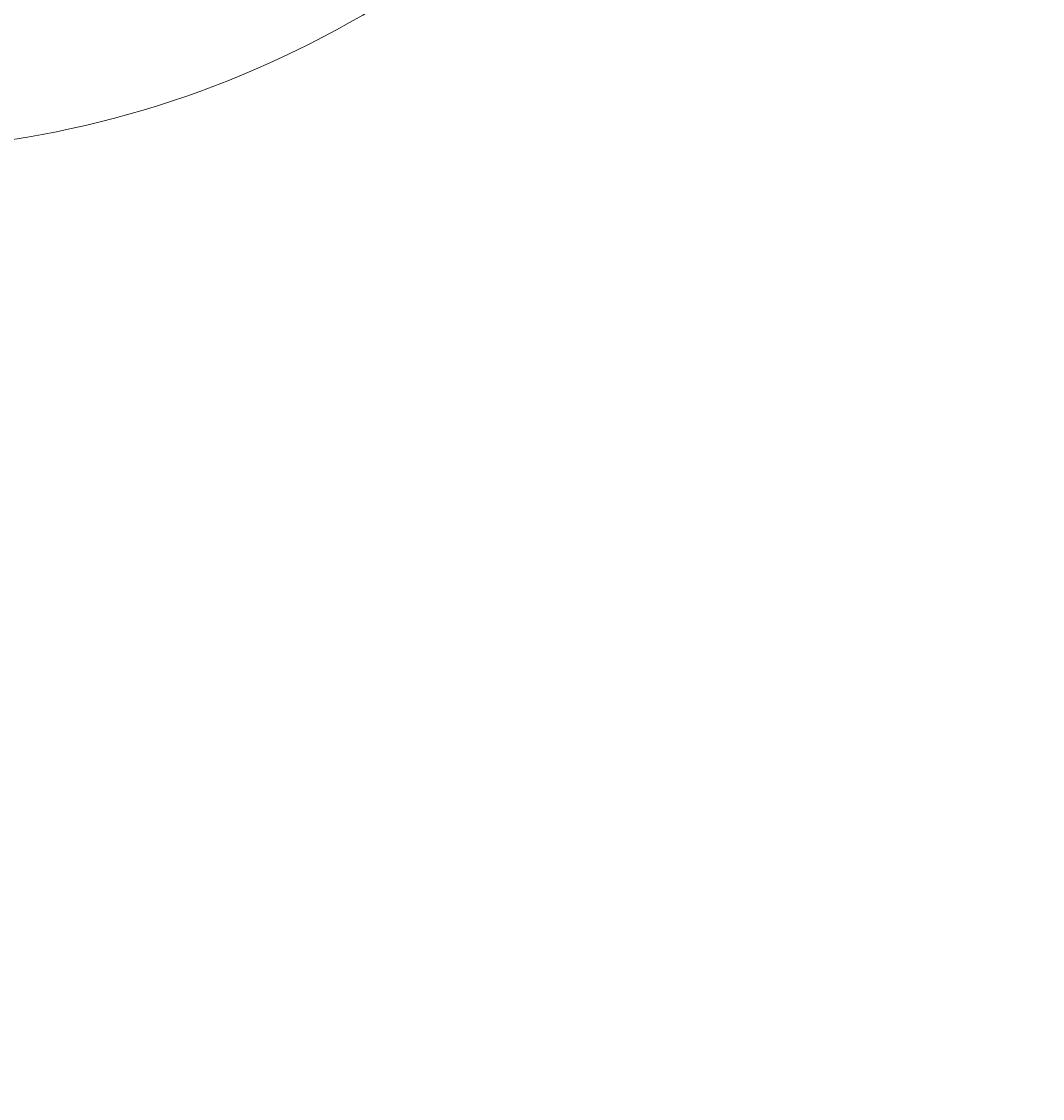
# Model space of a CAD drawing. Units: inches. Extents: x 1962 to 2771, y 1245 to 2660.
# Tile 65 of 114: x 2523 to 2551, y 2062 to 2091. Entities that reach past the tile are written whole.
import ezdxf

# ---------------------------------------------------------------- set-up
doc = ezdxf.new("R2010")
doc.units = ezdxf.units.IN
doc.layers.add('A-ANNO-DIMS', color=2, linetype='Continuous', lineweight=18)
doc.layers.add('A-DOOR', color=3, linetype='Continuous', lineweight=18)
doc.styles.get("Standard").update_dxf_attribs({"font": 'arial.ttf'})
doc.dimstyles.get("Standard").update_dxf_attribs({"dimtxt": 0.18, "dimasz": 0.18, "dimexe": 0.18, "dimexo": 0.0625, "dimgap": 0.09, "dimtad": 0, "dimtih": 1, "dimtoh": 1, "dimdec": 4, "dimzin": 0, "dimdsep": 46, "dimtxsty": 'Standard', "dimcen": 0.09, "dimadec": 0, "dimazin": 0, "dimtfac": 1, "dimtdec": 4, "dimtofl": 0, "dimtmove": 0, "dimatfit": 3, "dimfxl": 1, "dimtolj": 1, "dimtzin": 0, "dimarcsym": 0})

# ---------------------------------------------------------------- blocks, each defined once
blk = doc.blocks.new('*D40')
at = {"layer": 'A-ANNO-DIMS', "color": 0, "lineweight": -2, "transparency": 16777216}
for p, q in [((2072.02, 2033.906), (2072.02, 2583.474)), ((2660.807, 2524.406), (2660.807, 2583.474)), ((2072.2, 2583.294), (2366.02, 2583.294)), ((2660.627, 2583.294), (2366.808, 2583.294))]:
    blk.add_line(p, q, dxfattribs=at)
at = {"layer": 'A-ANNO-DIMS', "color": 0, "transparency": 16777216}
for points in [[(2072.2, 2583.324), (2072.2, 2583.264), (2072.02, 2583.294)], [(2660.627, 2583.324), (2660.627, 2583.264), (2660.807, 2583.294)]]:
    blk.add_solid(points, dxfattribs=at)
at = {"layer": 'Defpoints', "color": 0, "transparency": 16777216}
for p in [(2660.807, 2583.294), (2660.807, 2524.344), (2072.02, 2033.844)]:
    blk.add_point(p, dxfattribs=at)
at = {"layer": 'A-ANNO-DIMS', "color": 0, "transparency": 16777216, "insert": (2366.414, 2583.294), "char_height": 0.18, "attachment_point": 5}
blk.add_mtext('\\A1;588.8', dxfattribs=at)

msp = doc.modelspace()

# ---------------------------------------------------------------- linework, layer by layer
at = {"layer": 'A-DOOR'}
msp.add_arc((2518.9529, 2114.3027), 27.1044, 250.84069, 360, dxfattribs=at)

# ---------------------------------------------------------------- dimensions: what is measured, and where the dimension line sits
at = {"layer": 'A-ANNO-DIMS'}
dim = msp.add_linear_dim(base=(2660.8074, 2583.2937), p1=(2072.0204, 2033.8437), p2=(2660.8074, 2524.3437), dimstyle='Standard', override={"dimdec": 1, "dimlfac": 1, "dimrnd": 0, "dimzin": 0, "dimdsep": 46, "dimlunit": 2}, dxfattribs=at)
dim.commit()
dim.dimension.update_dxf_attribs({"geometry": '*D40', "text_midpoint": (2366.4139, 2583.2937)})

doc.saveas('drawing.dxf')
